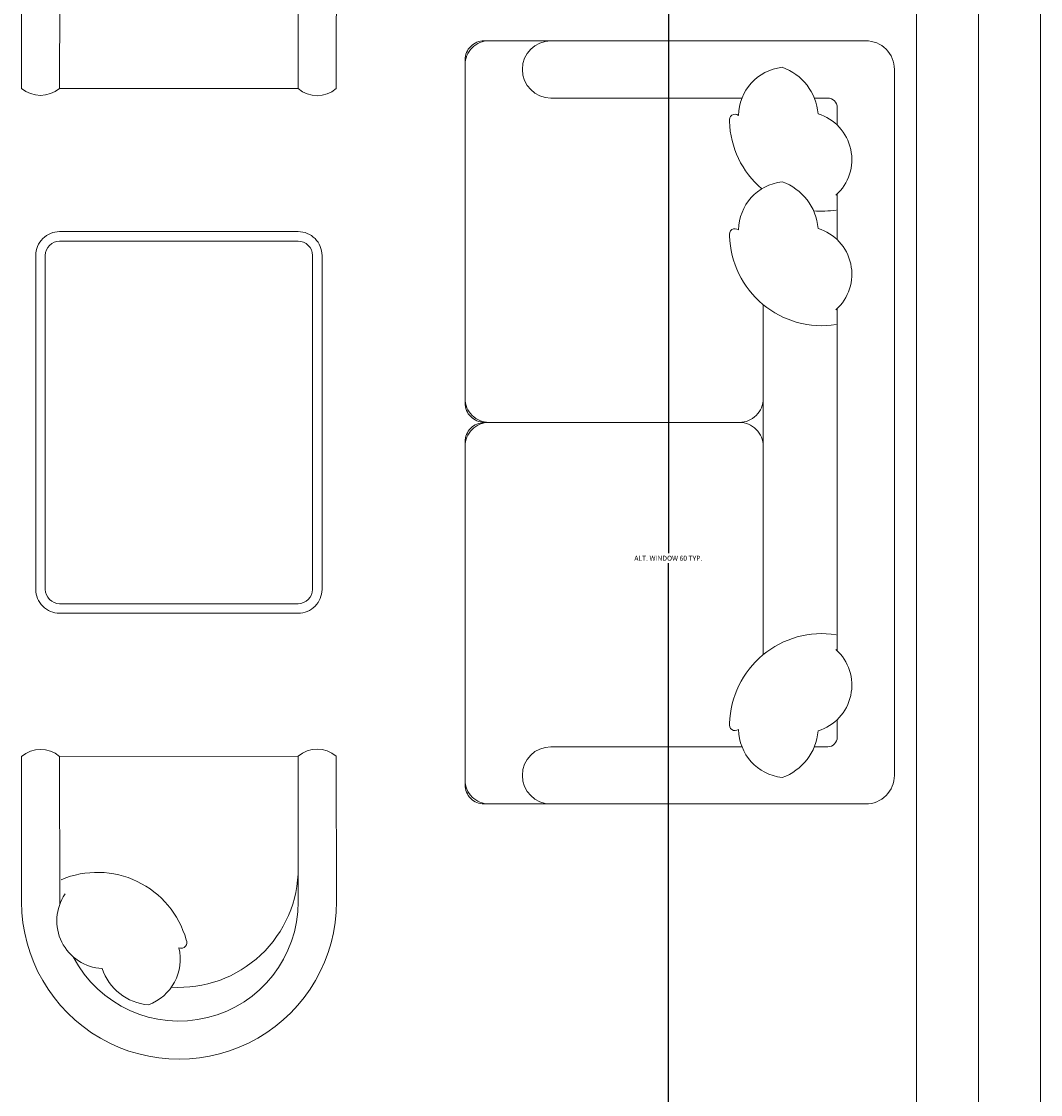
# Model space of a CAD drawing. Units: inches. Extents: x 1885 to 2748, y 783 to 2421.
# Tile 104 of 117: x 2581 to 2618, y 1907 to 1946. Entities that reach past the tile are written whole.
import ezdxf

# ---------------------------------------------------------------- set-up
doc = ezdxf.new("R2010")
doc.units = ezdxf.units.IN
for name, color, linetype, lineweight in [('A-ANNO-DIMS', 2, 'Continuous', 18), ('A-FURN', 8, 'Continuous', 13), ('A-GLAZ', 181, 'Continuous', 18)]:
    doc.layers.add(name, color=color, linetype=linetype, lineweight=lineweight)
doc.styles.get("Standard").update_dxf_attribs({"font": 'arial.ttf'})
doc.dimstyles.get("Standard").update_dxf_attribs({"dimtxt": 0.18, "dimasz": 0.18, "dimexe": 0.18, "dimexo": 0.0625, "dimgap": 0.09, "dimtad": 0, "dimtih": 1, "dimtoh": 1, "dimdec": 4, "dimzin": 0, "dimdsep": 46, "dimtxsty": 'Standard', "dimcen": 0.09, "dimadec": 0, "dimazin": 0, "dimtfac": 1, "dimtdec": 4, "dimtofl": 0, "dimtmove": 0, "dimatfit": 3, "dimfxl": 1, "dimtolj": 1, "dimtzin": 0, "dimarcsym": 0})

# ---------------------------------------------------------------- blocks, each defined once
blk = doc.blocks.new('A$C1352')
at = {"color": 0}
for points in [[(0.0027, 0.053), (0.0027, 0.553, -0.414214), (0.0527, 0.603), (0.7527, 0.603, -0.414214), (0.8027, 0.553), (0.8027, 0.053, -0.414214), (0.7527, 0.003), (0.0527, 0.003, -0.414214)], [(0.0227, 0.053), (0.0227, 0.553, -0.414214), (0.0527, 0.583), (0.7527, 0.583, -0.414214), (0.7827, 0.553), (0.7827, 0.053, -0.414214), (0.7527, 0.023), (0.0527, 0.023, -0.414214)]]:
    blk.add_lwpolyline(points, format="xyb", close=True, dxfattribs=at)
blk = doc.blocks.new('CHAIR-LOUNGE')
blk.add_line((1.388, 5.701), (1.383, 10.98))
at = {"ltscale": 0.03}
blk.add_lwpolyline([(1.383, 10.98, 0.369229), (-0.002, 10.979), (0.003, 5.7, 1), (11.423, 5.711), (11.418, 10.99, 0.369229), (10.034, 10.988)], format="xyb", close=True, dxfattribs=at)
blk.add_lwpolyline([(1.877, 3.707, 0.785087), (10.039, 5.71), (10.034, 10.988)], format="xyb")
for centre, radius, start, end in [((2.748, 3.424), 3.35, 15.7143, 112.9857), ((5.712, 6.928), 4.326, 266.342, 0.0539), ((3.014, 5.016), 1.734, 145.8599, 267.0078), ((5.713, 5.706), 4.326, 180.0539, 181.1464), ((5.792, 4.23), 0.207, 246.2577, 29.3762), ((3.979, 3.63), 1.778, 290.5305, 13.3597), ((4.772, 3.909), 1.951, 198.6466, 265.0001)]:
    blk.add_arc(centre, radius, start, end)
blk = doc.blocks.new('WIN-60-ALT')
for p, q in [((0.004, 59.998), (4.504, 59.998)), ((0.004, 59.998), (0.004, -0.002)), ((4.504, 59.998), (2.254, 59.998)), ((2.254, 59.998), (2.254, -0.002)), ((4.504, -0.002), (4.504, 59.998)), ((4.504, -0.002), (0.004, -0.002)), ((2.254, -0.002), (4.504, -0.002))]:
    blk.add_line(p, q)
blk = doc.blocks.new('*D17')
at = {"layer": 'A-ANNO-DIMS', "color": 0, "lineweight": -2, "transparency": 16777216}
for p, q in [((2613.711, 1956.755), (2604.594, 1956.755)), ((2604.774, 1956.575), (2604.774, 1926.938)), ((2604.774, 1896.935), (2604.774, 1926.572)), ((2613.711, 1896.755), (2604.594, 1896.755))]:
    blk.add_line(p, q, dxfattribs=at)
at = {"layer": 'A-ANNO-DIMS', "color": 0, "transparency": 16777216}
for points in [[(2604.744, 1956.575), (2604.804, 1956.575), (2604.774, 1956.755)], [(2604.744, 1896.935), (2604.804, 1896.935), (2604.774, 1896.755)]]:
    blk.add_solid(points, dxfattribs=at)
at = {"layer": 'Defpoints', "color": 0, "transparency": 16777216}
for p in [(2604.774, 1956.755), (2613.774, 1956.755), (2613.774, 1896.755)]:
    blk.add_point(p, dxfattribs=at)
at = {"layer": 'A-ANNO-DIMS', "color": 0, "transparency": 16777216, "insert": (2604.774, 1926.755), "char_height": 0.18, "attachment_point": 5}
blk.add_mtext('\\A1;ALT. WINDOW 60 TYP.', dxfattribs=at)

msp = doc.modelspace()

# ---------------------------------------------------------------- linework, layer by layer
at = {"layer": 'A-FURN'}
for p, q in [((2607.444, 1943.447), (2600.517, 1943.447)), ((2610.071, 1943.447), (2610.553, 1943.447)), ((2610.899, 1943.101), (2610.899, 1942.465)), ((2610.899, 1938.311), (2610.899, 1939.967)), ((2610.899, 1938.947), (2610.899, 1938.311)), ((2610.899, 1923.397), (2610.899, 1935.812)), ((2610.899, 1920.262), (2610.899, 1920.899)), ((2600.517, 1919.916), (2607.444, 1919.916)), ((2610.071, 1919.916), (2610.553, 1919.916))]:
    msp.add_line(p, q, dxfattribs=at)
at = {"layer": 'A-FURN', "ltscale": 0.03}
msp.add_lwpolyline([(2598.095, 1931.673, 0.414214), (2597.403, 1930.981), (2597.403, 1918.532, 0.414214), (2598.095, 1917.84), (2611.937, 1917.84, 0.414214), (2612.975, 1918.878), (2612.975, 1944.486, 0.414214), (2611.937, 1945.524), (2598.095, 1945.524, 0.414214), (2597.403, 1944.832), (2597.403, 1932.382, 0.414214), (2598.095, 1931.69)], format="xyb", dxfattribs=at)
at = {"layer": 'A-FURN'}
for points in [[(2608.217, 1935.951), (2608.217, 1932.547, -0.414214), (2607.352, 1931.682), (2598.268, 1931.682, -0.414214), (2597.403, 1932.547), (2597.403, 1944.659, -0.414214), (2598.268, 1945.524)], [(2608.217, 1923.847), (2608.217, 1930.817, 0.414214), (2607.352, 1931.682), (2598.268, 1931.682, 0.414214), (2597.403, 1930.817), (2597.403, 1918.705, 0.414214), (2598.268, 1917.84)]]:
    msp.add_lwpolyline(points, format="xyb", dxfattribs=at)
msp.add_lwpolyline([(2608.217, 1935.951), (2608.217, 1923.258)], dxfattribs=at)
for centre, radius, start, end in [((2600.517, 1944.486), 1.038, 90, 180), ((2600.517, 1944.486), 1.038, 180, 270), ((2609.098, 1942.795), 1.778, 96.4279, 179.257), ((2608.261, 1942.718), 1.951, 4.5439, 70.8974), ((2610.553, 1943.101), 0.346, 0, 90), ((2610.553, 1943.101), 0.346, 0, 90), ((2607.194, 1942.655), 0.207, 52.155, 195.2735), ((2609.696, 1941.216), 1.734, 311.7572, 72.9051), ((2610.342, 1942.694), 3.35, 181.6116, 229.376), ((2609.098, 1938.641), 1.778, 96.4279, 179.257), ((2608.261, 1938.564), 1.951, 4.5439, 70.8974), ((2610.342, 1942.694), 3.35, 264.881, 278.883), ((2607.194, 1938.501), 0.207, 52.155, 195.2735), ((2609.696, 1937.061), 1.734, 311.7572, 72.9051), ((2610.342, 1938.54), 3.35, 181.6116, 278.883), ((2610.342, 1920.669), 3.35, 81.117, 178.3884), ((2609.696, 1922.148), 1.734, 287.0949, 48.2428), ((2607.194, 1920.709), 0.207, 164.7265, 307.845), ((2609.098, 1920.568), 1.778, 180.743, 263.5721), ((2608.261, 1920.645), 1.951, 289.1026, 355.4561), ((2610.553, 1920.262), 0.346, 270, 0), ((2600.517, 1918.878), 1.038, 90, 180), ((2600.517, 1918.878), 1.038, 180, 270)]:
    msp.add_arc(centre, radius, start, end, dxfattribs=at)

# ---------------------------------------------------------------- block references
at = {"layer": 'A-FURN', "extrusion": (0, 0, -1), "zscale": -1, "rotation": 180}
msp.add_blockref('CHAIR-LOUNGE', (-2581.313, 1954.778), dxfattribs=at)
at = {"layer": 'A-FURN', "ltscale": 0.03, "xscale": 17.30251319894821, "yscale": 17.30251319894821, "zscale": 17.30251319894821, "rotation": 270}
msp.add_blockref('A$C1352', (2581.779, 1938.649), dxfattribs=at)
at = {"layer": 'A-FURN'}
msp.add_blockref('CHAIR-LOUNGE', (2581.313, 1908.586), dxfattribs=at)
at = {"layer": 'A-GLAZ'}
msp.add_blockref('WIN-60-ALT', (2613.77, 1896.757), dxfattribs=at)

# ---------------------------------------------------------------- dimensions: what is measured, and where the dimension line sits
at = {"layer": 'A-ANNO-DIMS'}
dim = msp.add_linear_dim(base=(2604.774, 1956.755), p1=(2613.774, 1896.755), p2=(2613.774, 1956.755), angle=90, text='ALT. WINDOW <> TYP.', dimstyle='Standard', override={"dimdec": 0, "dimlfac": 1, "dimrnd": 0, "dimzin": 0, "dimdsep": 46, "dimlunit": 2}, dxfattribs=at)
dim.commit()
dim.dimension.update_dxf_attribs({"geometry": '*D17', "text_midpoint": (2604.774, 1926.755)})

doc.saveas('drawing.dxf')
